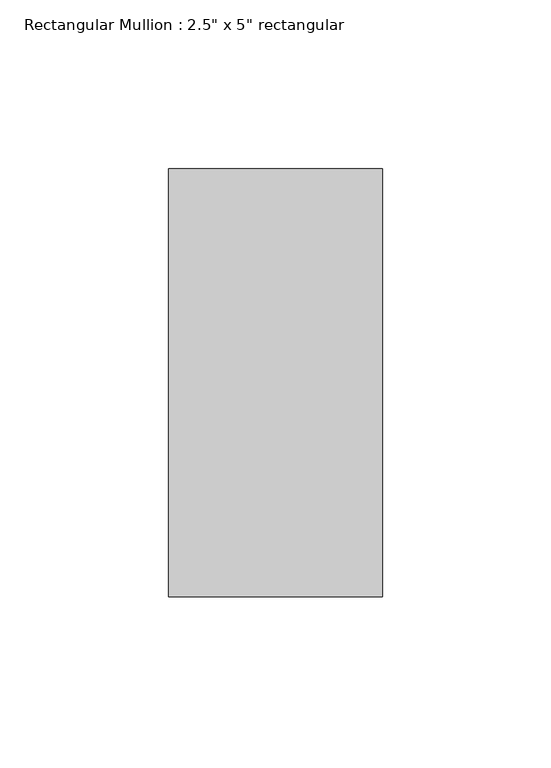
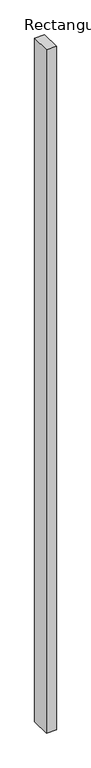
"""IFC4 building model written with IfcOpenShell, lengths in millimetres: member geometry."""

from ifc_helpers import new_model, si_unit, frame, origin, place, context, project, spatial, polyline, outline, extrude, source, transform, mapped, element, save


def member_d6d4b2c2(model_context):
    return source(origin(), model_context, "Body", "SweptSolid", [
        extrude(outline(polyline([(0.0, 63.5), (0.0, -63.5), (-63.5, -63.5), (-63.5, 63.5), (0.0, 63.5)])), frame((0.0, 0.0, -4559.3), z_axis=(0.0, 0.0, 1.0), x_axis=(1.0, 0.0, 0.0)), (0.0, 0.0, 1.0), 4559.3),
    ])


if __name__ == "__main__":
    model = new_model("IFC4")
    model_context = context("Model", 3, world=origin())
    ifc_project = project(units=[si_unit("LENGTHUNIT", "METRE", prefix="MILLI")], contexts=[model_context])
    site = spatial("IfcSite", under=ifc_project)
    building = spatial("IfcBuilding", under=site)
    placement = place(None, origin())
    member_shape = member_d6d4b2c2(model_context)
    element("IfcMember", 1, ObjectType="Rectangular Mullion : 2.5\" x 5\" rectangular", at=placement, inside=building, context=model_context, shape_type="MappedRepresentation", body=[
        mapped(member_shape, transform((0.0, 0.0, 0.0), x_axis=(1.0, 0.0, 0.0), y_axis=(0.0, 1.0, 0.0), z_axis=(0.0, 0.0, 1.0))),
    ])
    save(model, "model.ifc")

# Revit data of these elements
# Type "Rectangular Mullion : 2.5\" x 5\" rectangular"
#   built-in parameter 1007304 = 0.416667 (stored number, unit not read)
#   built-in parameter 1007301 = 0.104167 (stored number, unit not read)
#   built-in parameter 1007300 = 0.104167 (stored number, unit not read)
# Element 1 (IfcMember, "Rectangular Mullion : 2.5\" x 5\" rectangular")
#   Materials on its faces: "Aluminum"
# Materials
#   "Aluminum": class "Metal", colour RGB 247 247 247, transparency 0, Description = "Aluminum 6061", Cost = 0
